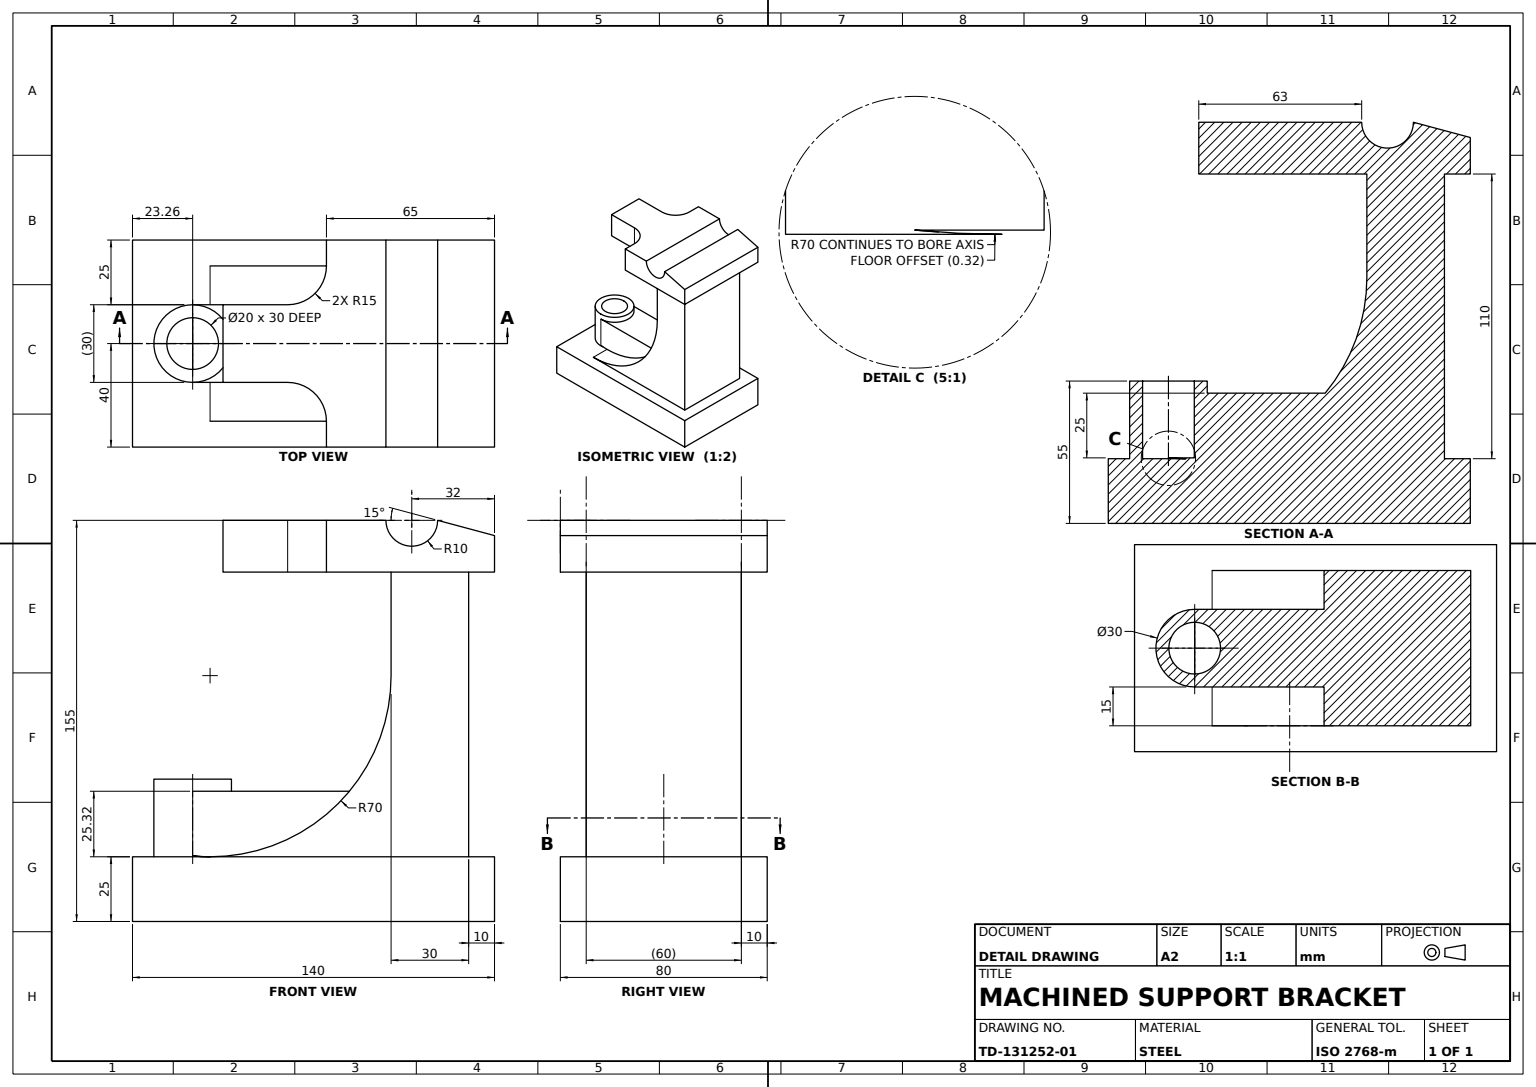
from build123d import *

# Parameters (mm, degrees)
BRACKET_BODY_DEPTH          = 40
BASE_RECESS_SKETCH_W        = 10
BASE_RECESS_SKETCH_H        = 110
BASE_RECESS_CUT_DEPTH       = 207.215906273
CRADLE_GROOVE_R15_DEPTH     = 80
TOP_CHAMFER_CUT_15DEG_DEPTH = 80
PIN_BOSS_SKETCH_R           = 15
PIN_BOSS_SKETCH_R_2         = 10
PIN_BOSS_DEPTH              = 55
CURVED_WEB_DEPTH            = 15
PIN_START                   = -25
PIN_BORE_SKETCH_R           = 10
PIN_BORE_20_DEPTH           = 25


with BuildPart() as part:
    # Bracket Profile Sketch → Bracket Body (new, symmetric)
    with BuildSketch(Plane.XY):
        with BuildLine():
            Line((-40, 25), (60, 25))
            Line((60, 25), (60, 135))
            Line((60, 135), (70, 135))
            Line((70, 135), (70, 155))
            Line((70, 155), (48, 155))
            ThreePointArc((48, 155), (38, 145), (28, 155))
            Line((28, 155), (-35, 155))
            Line((-35, 155), (-35, 135))
            Line((-35, 135), (30, 135))
            Line((30, 135), (30, 95))
            ThreePointArc((30, 95), (9.497474683, 45.502525317), (-40, 25))
        make_face()
        Polygon((-70, 25), (-70, 0), (0, 0), (70, 0), (70, 25), align=None)
    extrude(amount=BRACKET_BODY_DEPTH, both=True)

    # Base Recess Sketch → Base Recess Cut (cut, through all)
    with BuildSketch(Plane(origin=(60, 0, 0), x_dir=(0, 0, -1), z_dir=(1, 0, 0))):
        with Locations((35, 80)):
            Rectangle(BASE_RECESS_SKETCH_W, BASE_RECESS_SKETCH_H)
        with Locations((-35, 80)):
            Rectangle(BASE_RECESS_SKETCH_W, BASE_RECESS_SKETCH_H)
    extrude(amount=-BASE_RECESS_CUT_DEPTH, mode=Mode.SUBTRACT)

    # Cradle Groove Sketch → Cradle Groove R15 (cut)
    with BuildSketch(Plane(origin=(0, 155, 0), x_dir=(1, 0, 0), z_dir=(0, 1, 0))):
        with BuildLine():
            Line((-35, 40), (-35, 15))
            Line((-35, 15), (-10, 15))
            ThreePointArc((-10, 15), (0.606601718, 19.393398282), (5, 30))
            Line((5, 30), (5, 40))
            Line((5, 40), (-35, 40))
        make_face()
        with BuildLine():
            Line((-10, -15), (-35, -15))
            Line((-35, -15), (-35, -40))
            Line((-35, -40), (5, -40))
            Line((5, -40), (5, -30))
            ThreePointArc((5, -30), (0.606601718, -19.393398282), (-10, -15))
        make_face()
    extrude(amount=-CRADLE_GROOVE_R15_DEPTH, mode=Mode.SUBTRACT)

    # Top Chamfer Sketch → Top Chamfer Cut 15deg (cut)
    with BuildSketch(Plane.XY.offset(40)):
        Polygon((48, 155), (70, 149.105117767), (70, 155), align=None)
    extrude(amount=-TOP_CHAMFER_CUT_15DEG_DEPTH, mode=Mode.SUBTRACT)

    # Pin Boss Sketch → Pin Boss (add)
    with BuildSketch(Plane(origin=(0, 0, 0), x_dir=(1, 0, 0), z_dir=(0, 1, 0))):
        with Locations(Location((-46.735177318, 0, 0), (0, 0, 63.319698917))):
            Circle(PIN_BOSS_SKETCH_R)
        with Locations(Location((-46.735177318, 0, 0), (0, 0, 47.660850918))):
            Circle(PIN_BOSS_SKETCH_R_2, mode=Mode.SUBTRACT)
    extrude(amount=PIN_BOSS_DEPTH)

    # Curved Web Sketch → Curved Web (add, symmetric)
    with BuildSketch(Plane.XY):
        with BuildLine():
            Line((-46.735177318, 25.324772074), (-46.735177318, 50.324772074))
            Line((-46.735177318, 50.324772074), (13.889924938, 50.324772074))
            ThreePointArc((13.889924938, 50.324772074), (-13.314000754, 30.286342676), (-46.735177318, 25.324772074))
        make_face()
    extrude(amount=CURVED_WEB_DEPTH, both=True)

    # Pin Bore Sketch → Pin Bore Ø20 (cut)
    with BuildSketch(Plane(origin=(0, 50.324772074, 0), x_dir=(1, 0, 0), z_dir=(0, 1, 0)).offset(PIN_START)):
        with Locations(Location((-46.735177318, 0, 0), (0, 0, 270))):
            Circle(PIN_BORE_SKETCH_R)
    extrude(amount=PIN_BORE_20_DEPTH, mode=Mode.SUBTRACT)


solid = part.part
